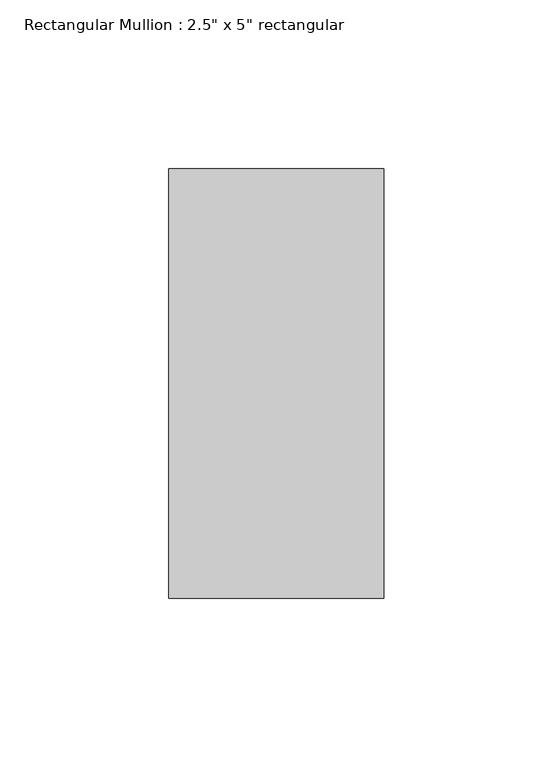
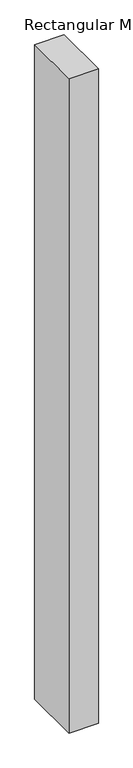
"""IFC4 building model written with IfcOpenShell, lengths in millimetres: member geometry."""

from ifc_helpers import new_model, si_unit, frame, origin, place, context, project, spatial, polyline, outline, extrude, source, transform, mapped, element, save


def member_fc57e1ce(model_context):
    return source(origin(), model_context, "Body", "SweptSolid", [
        extrude(outline(polyline([(0.0, 63.5), (0.0, -63.5), (-63.5, -63.5), (-63.5, 63.5), (0.0, 63.5)])), frame((0.0, 0.0, -1486.9744191), z_axis=(0.0, 0.0, 1.0), x_axis=(1.0, 0.0, 0.0)), (0.0, 0.0, 1.0), 1486.9744191),
    ])


if __name__ == "__main__":
    model = new_model("IFC4")
    model_context = context("Model", 3, world=origin())
    ifc_project = project(units=[si_unit("LENGTHUNIT", "METRE", prefix="MILLI")], contexts=[model_context])
    site = spatial("IfcSite", under=ifc_project)
    building = spatial("IfcBuilding", under=site)
    placement = place(None, origin())
    member_shape = member_fc57e1ce(model_context)
    element("IfcMember", 1, ObjectType="Rectangular Mullion : 2.5\" x 5\" rectangular", at=placement, inside=building, context=model_context, shape_type="MappedRepresentation", body=[
        mapped(member_shape, transform((0.0, 0.0, 0.0), x_axis=(1.0, 0.0, 0.0), y_axis=(0.0, 1.0, 0.0), z_axis=(0.0, 0.0, 1.0))),
    ])
    save(model, "model.ifc")

# Revit data of these elements
# Type "Rectangular Mullion : 2.5\" x 5\" rectangular"
#   built-in parameter 1007304 = 0.416667 (stored number, unit not read)
#   built-in parameter 1007301 = 0.104167 (stored number, unit not read)
#   built-in parameter 1007300 = 0.104167 (stored number, unit not read)
# Element 1 (IfcMember, "Rectangular Mullion : 2.5\" x 5\" rectangular")
#   Materials on its faces: "Aluminum"
# Materials
#   "Aluminum": class "Metal", colour RGB 247 247 247, transparency 0, Description = "Aluminum 6061", Cost = 0
